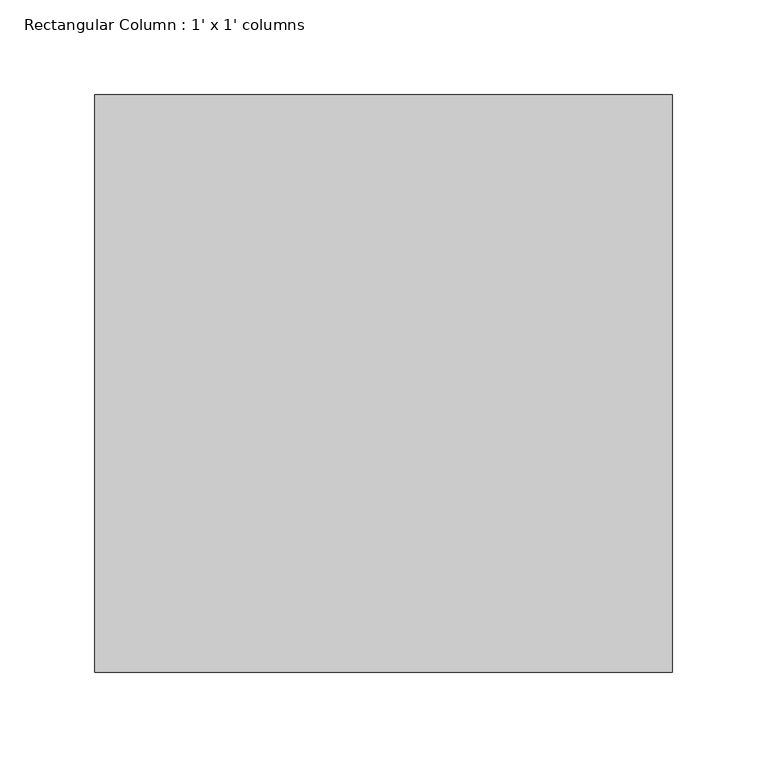
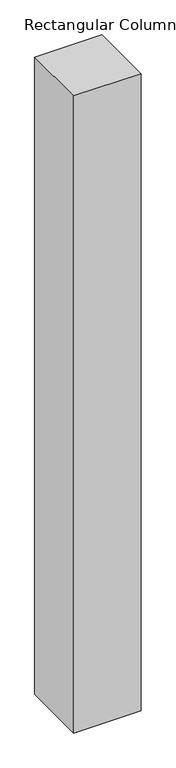
"""IFC4 building model written with IfcOpenShell, lengths in millimetres: column geometry, Rectangular Column : 1' x 1' columns."""

from ifc_helpers import new_model, si_unit, frame, origin, place, context, project, spatial, polyline, outline, extrude, source, transform, mapped, element, save


def rectangular_column_1_x_1_columns_77852fec(model_context):
    return source(origin(), model_context, "Body", "SweptSolid", [
        extrude(outline(polyline([(152.4, 152.4), (152.4, -152.4), (-152.4, -152.4), (-152.4, 152.4), (152.4, 152.4)])), frame((0.0, 0.0, 304.8), z_axis=(0.0, 0.0, 1.0), x_axis=(1.0, 0.0, 0.0)), (0.0, 0.0, 1.0), 3048.0),
    ])


if __name__ == "__main__":
    model = new_model("IFC4")
    model_context = context("Model", 3, world=origin())
    ifc_project = project(units=[si_unit("LENGTHUNIT", "METRE", prefix="MILLI")], contexts=[model_context])
    site = spatial("IfcSite", under=ifc_project)
    building = spatial("IfcBuilding", under=site)
    placement = place(None, origin())
    rectangular_column_1_x_1_columns_shape = rectangular_column_1_x_1_columns_77852fec(model_context)
    element("IfcColumn", 1, ObjectType="Rectangular Column : 1' x 1' columns", at=placement, inside=building, context=model_context, shape_type="MappedRepresentation", body=[
        mapped(rectangular_column_1_x_1_columns_shape, transform((0.0, 0.0, 0.0), x_axis=(1.0, 0.0, 0.0), y_axis=(0.0, 1.0, 0.0), z_axis=(0.0, 0.0, 1.0))),
    ])
    save(model, "model.ifc")

# Revit data of these elements
# Type "Rectangular Column : 1' x 1' columns"
#   Assembly Code = "B1010200"
#   Depth = 1' - 0"
#   Offset Base = 0' - 0"
#   Offset Top = 0' - 0"
#   Width = 1' - 0"
#   Material = OUTER WALL 9"
# Element 1 (IfcColumn, "Rectangular Column : 1' x 1' columns")
#   Materials on its faces: "OUTER WALL 9\""
# Materials
#   "OUTER WALL 9\"": class "Generic", colour RGB 120 120 120, transparency 0, Cost = 0
